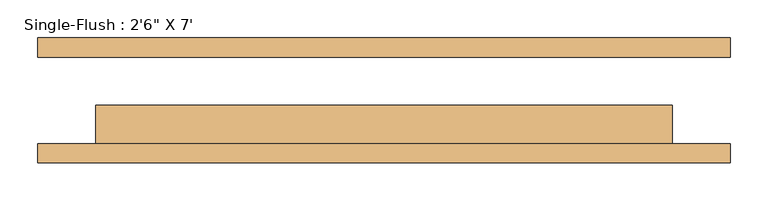
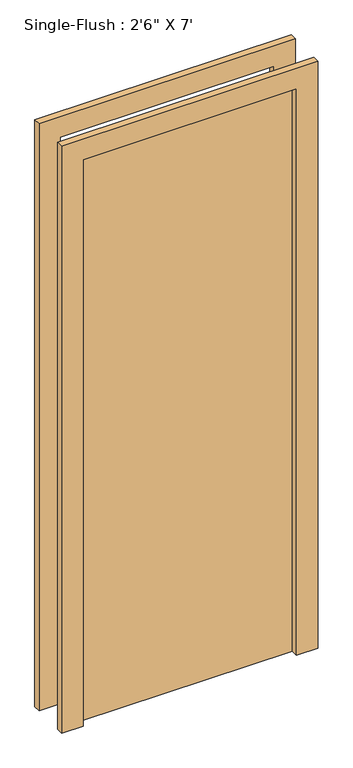
"""IFC4 building model written with IfcOpenShell, lengths in millimetres: door geometry."""

from ifc_helpers import new_model, si_unit, frame, origin, origin_with_axes, place, context, project, spatial, polyline, outline, extrude, source, transform, mapped, element, save


def door_78caadf7(model_context):
    return source(origin(), model_context, "Body", "SweptSolid", [
        extrude(outline(polyline([(2209.8, -457.2), (0.0, -457.2), (0.0, -381.0), (2133.6, -381.0), (2133.6, 381.0), (0.0, 381.0), (0.0, 457.2), (2209.8, 457.2), (2209.8, -457.2)])), frame((0.0, -82.55, 0.0), z_axis=(0.0, 1.0, 0.0), x_axis=(0.0, 0.0, 1.0)), (0.0, 0.0, 1.0), 25.4),
        extrude(outline(polyline([(2209.8, 457.2), (2209.8, -457.2), (0.0, -457.2), (0.0, -381.0), (2133.6, -381.0), (2133.6, 381.0), (0.0, 381.0), (0.0, 457.2), (2209.8, 457.2)])), frame((0.0, 57.15, 0.0), z_axis=(0.0, 1.0, 0.0), x_axis=(0.0, 0.0, 1.0)), (0.0, 0.0, 1.0), 25.4),
        extrude(outline(polyline([(381.0, -6.35), (381.0, -57.15), (-381.0, -57.15), (-381.0, -6.35), (381.0, -6.35)])), origin_with_axes(), (0.0, 0.0, 1.0), 2133.6),
    ])


if __name__ == "__main__":
    model = new_model("IFC4")
    model_context = context("Model", 3, world=origin())
    ifc_project = project(units=[si_unit("LENGTHUNIT", "METRE", prefix="MILLI")], contexts=[model_context])
    site = spatial("IfcSite", under=ifc_project)
    building = spatial("IfcBuilding", under=site)
    placement = place(None, origin())
    door_shape = door_78caadf7(model_context)
    element("IfcDoor", 1, ObjectType="Single-Flush : 2'6\" X 7'", at=placement, inside=building, context=model_context, shape_type="MappedRepresentation", body=[
        mapped(door_shape, transform((0.0, 0.0, 0.0), x_axis=(1.0, 0.0, 0.0), y_axis=(0.0, 1.0, 0.0), z_axis=(0.0, 0.0, 1.0))),
    ])
    save(model, "model.ifc")

# Revit data of these elements
# Type "Single-Flush : 2'6\" X 7'"
#   Type Mark = "8"
#   Construction Type Id = "MDOOR"
#   Assembly Code = "C1020"
#   Analytic Construction = "Metal"
#   Thickness = 0' - 2"
#   Heat Transfer Coefficient (U) = 0.651978 BTU/(h·ft²·°F)
#   Height = 7' - 0"
#   Trim Projection Ext = 0' - 1"
#   Trim Projection Int = 0' - 1"
#   Trim Width = 0' - 3"
#   Width = 2' - 6"
#   Define Thermal Properties by = 1
#   Door Material = Door - Panel
#   Frame Material = Door - Frame
#   Visual Light Transmittance = 0
#   Solar Heat Gain Coefficient = 0
#   Function = (empty or 0)
#   Wall Closure = (empty or 0)
# Element 1 (IfcDoor, "Single-Flush : 2'6\" X 7'")
#   Materials on its faces: "Door - Frame", "Door - Panel"
# Materials
#   "Door - Panel": class "Wood", colour RGB 210 159 95, transparency 0, Cost = 0
#   "Door - Frame": colour RGB 118 70 51, transparency 0, Cost = 0
